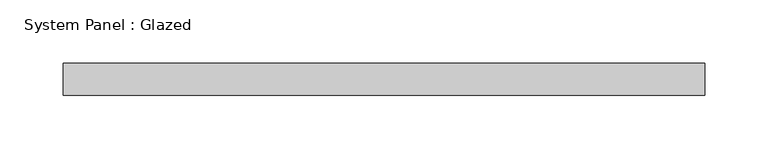
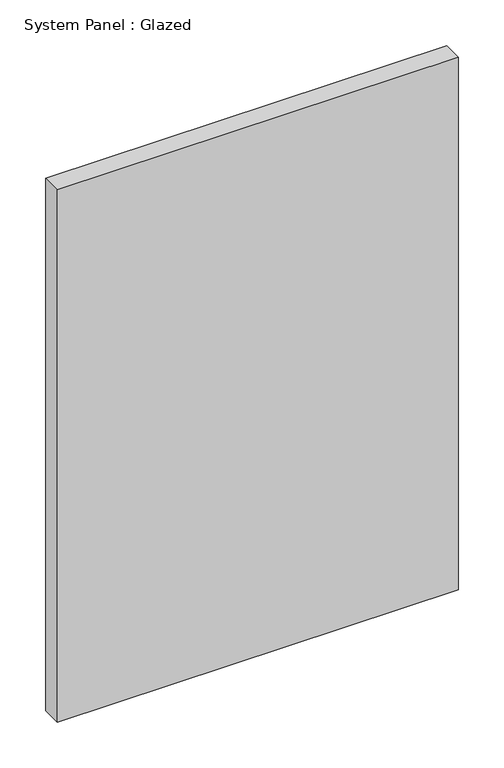
"""IFC4 building model written with IfcOpenShell, lengths in millimetres: plate geometry, System Panel : Glazed."""

from ifc_helpers import new_model, si_unit, origin, origin_with_axes, place, context, project, spatial, polyline, outline, extrude, source, transform, mapped, element, save


def system_panel_glazed_11c7b7b5(model_context):
    return source(origin(), model_context, "Body", "SweptSolid", [
        extrude(outline(polyline([(254.0, 19.05), (-254.0, 19.05), (-254.0, 44.45), (254.0, 44.45), (254.0, 19.05)])), origin_with_axes(), (0.0, 0.0, 1.0), 713.1032277),
    ])


if __name__ == "__main__":
    model = new_model("IFC4")
    model_context = context("Model", 3, world=origin())
    ifc_project = project(units=[si_unit("LENGTHUNIT", "METRE", prefix="MILLI")], contexts=[model_context])
    site = spatial("IfcSite", under=ifc_project)
    building = spatial("IfcBuilding", under=site)
    placement = place(None, origin())
    system_panel_glazed_shape = system_panel_glazed_11c7b7b5(model_context)
    element("IfcPlate", 1, ObjectType="System Panel : Glazed", at=placement, inside=building, context=model_context, shape_type="MappedRepresentation", body=[
        mapped(system_panel_glazed_shape, transform((0.0, 0.0, 0.0), x_axis=(1.0, 0.0, 0.0), y_axis=(0.0, 1.0, 0.0), z_axis=(0.0, 0.0, 1.0))),
    ])
    save(model, "model.ifc")

# Revit data of these elements
# Type "System Panel : Glazed"
#   Construction Type Id = "GSP4R"
#   Analytic Construction = "1/8 in Pilkington single glazing"
#   Visual Light Transmittance = 0.9
#   Solar Heat Gain Coefficient = 0.86
#   Heat Transfer Coefficient (U) = 1.18115 BTU/(h·ft²·°F)
#   Define Thermal Properties by = 1
# Element 1 (IfcPlate, "System Panel : Glazed")
#   Materials on its faces: "Glass"
# Materials
#   "Glass": class "Glass", colour RGB 0 128 192, transparency 0.75, Description = "Soda Lime Glass", Cost = 0
